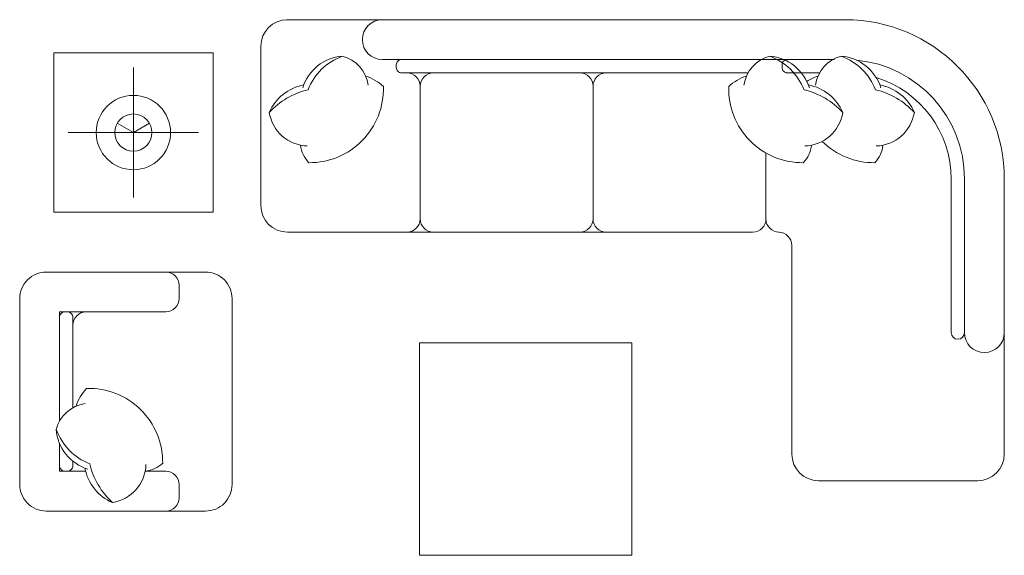
# Model space of a CAD drawing. Units: inches. Extents: x -317284 to 524, y -2236 to 1075.
# Tile 1 of 6: x -317284 to -313576, y -2236 to -219. Entities that reach past the tile are written whole.
import ezdxf

# ---------------------------------------------------------------- set-up
doc = ezdxf.new("R2010")
doc.units = ezdxf.units.IN
doc.header["$MEASUREMENT"] = 0
doc.layers.add('A-FURN', color=8, linetype='Continuous', lineweight=18)

# ---------------------------------------------------------------- blocks, each defined once
blk = doc.blocks.new('A$C714C64AF')
for p, q in [((3108.1, 2016.8, -5498.8), (1005.4, 2016.8, -5498.8)), ((908.1, 1916.8, -5498.8), (908.1, 1316.8, -5498.8)), ((1365.5, 1866.8, -5498.8), (2793.4, 1866.8, -5498.8)), ((3508.1, 1416.8, -5498.8), (3508.1, 838.6, -5498.8)), ((3558.1, 1416.8, -5498.8), (3558.1, 838.6, -5498.8)), ((3708.1, 1416.8, -5498.8), (3708.1, 838.6, -5498.8)), ((1008.1, 1216.8, -5498.8), (1458.1, 1216.8, -5498.8)), ((1558.1, 1216.8, -5498.8), (1458.1, 1216.8, -5498.8)), ((1558.1, 1216.8, -5498.8), (2760.4, 1216.8, -5498.8)), ((2209.2, 1216.8, -5498.8), (2109.2, 1216.8, -5498.8)), ((2908.1, 1166.8, -5498.8), (2908.1, 381, -5498.8)), ((3708.1, 838.6, -5498.8), (3708.1, 381, -5498.8)), ((3008.1, 281, -5498.8), (3608.1, 281, -5498.8))]:
    blk.add_line(p, q)
at = {"elevation": -5498.8}
for points in [[(128.1, 1891.8), (728.1, 1891.8), (728.1, 1291.8), (128.1, 1291.8)], [(2305.7, 800), (1505.6, 800), (1505.6, 0), (2305.7, 0)]]:
    blk.add_lwpolyline(points, close=True, dxfattribs=at)
for points in [[(939.9, 1667.3, -0.14773), (1086, 1753.2, -0.213343), (1215, 1879.3)], [(1065.8, 1760.1, -0.306663), (1215, 1879.3, -0.30633), (1312.4, 1770.4)], [(1456.3, 1816.8), (1438.2, 1816.8, -0.414214), (1418.2, 1836.8), (1418.2, 1846.8, -0.414214), (1438.2, 1866.8)], [(2669.7, 1866.8), (1883.5, 1866.8, 0.414214)], [(2974, 1760.1, 0.306663), (2824.8, 1879.3, 0.30633), (2727.4, 1770.4)], [(3068.1, 1866.8), (2752.9, 1866.8, 0.415492)], [(3099.9, 1667.3, 0.14773), (2953.8, 1753.2, 0.213343), (2824.8, 1879.3)], [(3013.4, 1866.8), (2891.1, 1866.8, 0.414214), (2871.1, 1846.8), (2871.1, 1836.8, 0.414214), (2891.1, 1816.8), (2963, 1816.8, 0.414214)], [(3243.3, 1760.1, 0.306663), (3094.2, 1879.3, 0.30633), (2996.8, 1770.4)], [(3369.3, 1667.3, 0.14773), (3223.1, 1753.2, 0.213343), (3094.2, 1879.3)], [(1058, 1544.3, 0.165541), (1088.9, 1478.3, 0.425989), (1369.7, 1764.7, 0.121523), (1303.1, 1804.2)], [(1458.1, 1816.8, -0.414214), (1508.1, 1766.8)], [(1558.1, 1816.8, 0.414214), (1508.1, 1766.8), (1508.1, 1266.8, 0.432452)], [(1558.1, 1816.8, 0.414214), (1508.1, 1766.8)], [(2109.2, 1816.8, -0.414214), (2159.2, 1766.8)], [(2209.2, 1816.8, 0.414214), (2159.2, 1766.8), (2159.2, 1266.8, 0.432452)], [(2209.2, 1816.8, 0.414214), (2159.2, 1766.8)], [(2981.8, 1544.3, -0.165541), (2950.9, 1478.3, -0.425989), (2670.1, 1764.7, -0.121523), (2736.8, 1804.2)], [(2964.2, 1784.6, -0.071865), (3006.1, 1804.2)], [(1083.2, 1541.3, -0.356772), (939.9, 1667.3, -0.249542), (1069.7, 1771.2)], [(2956.6, 1541.3, 0.356772), (3099.9, 1667.3, 0.249542), (2970.1, 1771.2)], [(3226, 1541.3, 0.356772), (3369.3, 1667.3, 0.249542), (3239.4, 1771.2)], [(3251.2, 1544.3, -0.165541), (3220.3, 1478.3, -0.200231), (3021.8, 1558.7)], [(150, 505), (150, 916.7), (550, 916.7, 0.414214), (600, 966.7), (600, 1016.7, 0.414214), (550, 1066.7)], [(150, 505), (150, 916.7), (550, 916.7, 0.414214), (600, 966.7), (600, 1016.7, 0.414214), (550, 1066.7)], [(150, 505), (150, 896.7, -0.414214), (170, 916.7), (180, 916.7, -0.414214), (200, 896.7), (200, 555.4, -0.729729)], [(250, 916.7, 0.414214), (200, 866.7)], [(472.5, 316.5, 0.165541), (538.6, 347.5, 0.425989), (252.1, 628.3, 0.121523), (212.7, 561.6)], [(256.7, 324.4, -0.306663), (137.6, 473.6, -0.30633), (246.4, 571)], [(349.5, 198.5, -0.14773), (263.6, 344.6, -0.213343), (137.6, 473.6)], [(150, 336.7), (150, 421.8, -0.414213)], [(200, 354.8), (200, 336.7, -0.414214), (180, 316.7), (170, 316.7, -0.414214), (150, 336.7)], [(475.6, 341.7, -0.356772), (349.5, 198.5, -0.249542), (245.7, 328.3)], [(472.5, 316.7), (550, 316.7, -0.414214), (600, 266.7), (600, 216.7, -0.414214), (550, 166.7)]]:
    blk.add_lwpolyline(points, format="xyb", dxfattribs=at)
for points in [[(1883.5, 1866.8), (2669.7, 1866.8)], [(428.1, 1836.8), (428.1, 1346.8)], [(1458.1, 1816.8), (2743, 1816.8)], [(2943.6, 1816.8), (3012.4, 1816.8)], [(428.1, 1591.8), (367.5, 1626.8)], [(428.1, 1591.8), (488.7, 1626.8)], [(183.1, 1591.8), (673.1, 1591.8)], [(428.1, 1591.8), (428.1, 1521.8)], [(2810.4, 1514.8), (2810.4, 1266.8)], [(248.3, 316.7), (150, 316.7), (150, 421.8)]]:
    blk.add_lwpolyline(points, dxfattribs=at)
blk.add_lwpolyline([(0, 266.7, 0.414214), (100, 166.7), (700, 166.7, 0.414214), (800, 266.7), (800, 966.7, 0.414214), (700, 1066.7), (100, 1066.7, 0.414214), (0, 966.7)], format="xyb", close=True, dxfattribs=at)
for radius in [140, 70]:
    blk.add_circle((428.1, 1591.8, -5498.8), radius)
for centre, radius, start, end in [((1008.1, 1916.8, -5498.8), 100, 90, 180), ((1365.5, 1941.8, -5498.8), 75, 90, 270), ((3108.1, 1416.8, -5498.8), 600, 0, 90), ((3108.1, 1416.8, -5498.8), 450, 0, 84.5853), ((3108.1, 1416.8, -5498.8), 400, 0, 72.9371), ((1008.1, 1316.8, -5498.8), 100, 180, 270), ((1458.1, 1266.8, -5498.8), 50, 270, 0), ((1458.1, 1266.8, -5498.8), 50, 270, 0), ((1558.1, 1266.8, -5498.8), 50, 180, 270), ((1558.1, 1266.8, -5498.8), 50, 180, 270), ((2109.2, 1266.8, -5498.8), 50, 270, 0), ((2109.2, 1266.8, -5498.8), 50, 270, 0), ((2209.2, 1266.8, -5498.8), 50, 180, 270), ((2209.2, 1266.8, -5498.8), 50, 180, 270), ((2760.4, 1266.8, -5498.8), 50, 270, 0), ((2760.4, 1266.8, -5498.8), 50, 270, 0), ((2860.4, 1266.8, -5498.8), 50, 180, 270), ((2860.4, 1266.8, -5498.8), 50, 180, 270), ((2858.1, 1166.8, -5498.8), 50, 0, 90), ((3533.1, 838.6, -5498.8), 25, 180, 0), ((3633.1, 838.6, -5498.8), 75, 180, 0), ((3008.1, 381, -5498.8), 100, 180, 270), ((3608.1, 381, -5498.8), 100, 270, 0)]:
    blk.add_arc(centre, radius, start, end)

msp = doc.modelspace()

# ---------------------------------------------------------------- block references
at = {"layer": 'A-FURN'}
msp.add_blockref('A$C714C64AF', (-317283.89, -2235.63), dxfattribs=at)

doc.saveas('drawing.dxf')
